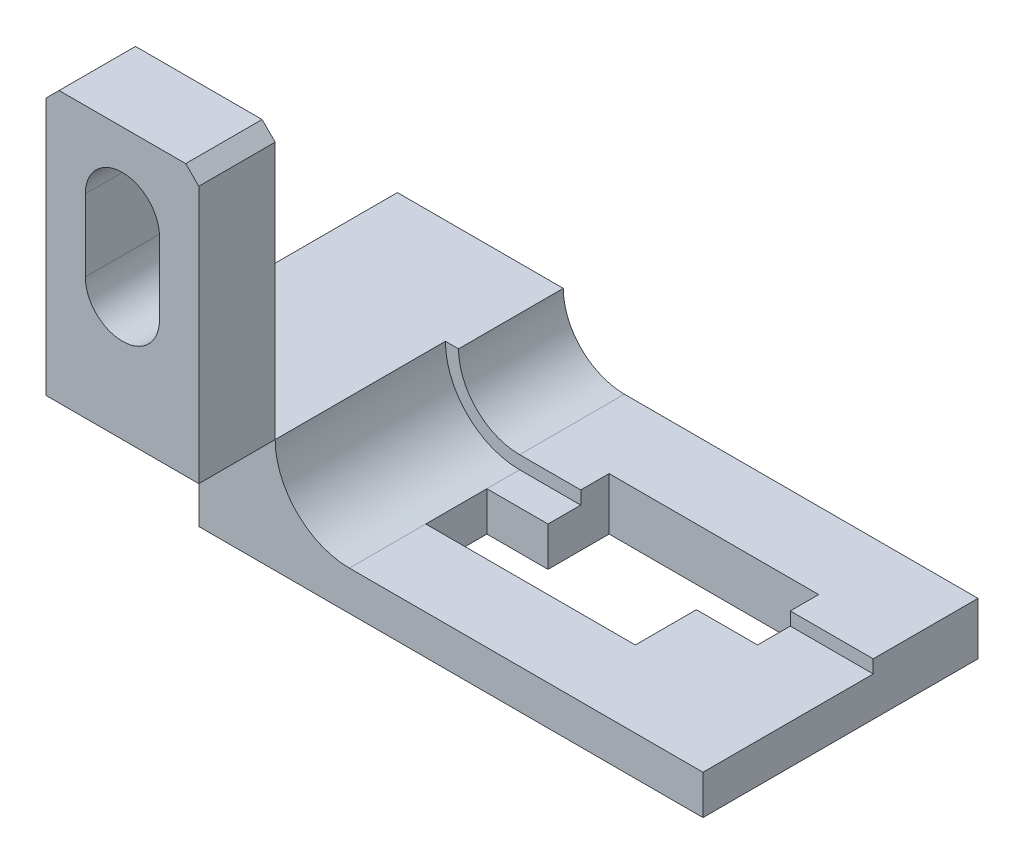
ISO-10303-21;
HEADER;
FILE_DESCRIPTION(('STEP AP214'),'2;1');
FILE_NAME('part.step','',(''),(''),'','','');
FILE_SCHEMA(('AUTOMOTIVE_DESIGN { 1 0 10303 214 1 1 1 1 }'));
ENDSEC;
DATA;
#1=APPLICATION_CONTEXT('core data for automotive mechanical design processes');
#2=APPLICATION_PROTOCOL_DEFINITION('international standard','automotive_design',2000,#1);
#3=PRODUCT_CONTEXT('',#1,'mechanical');
#4=PRODUCT('Part','Part','',(#3));
#5=PRODUCT_RELATED_PRODUCT_CATEGORY('part','',(#4));
#6=PRODUCT_DEFINITION_FORMATION('','',#4);
#7=PRODUCT_DEFINITION_CONTEXT('part definition',#1,'design');
#8=PRODUCT_DEFINITION('design','',#6,#7);
#9=PRODUCT_DEFINITION_SHAPE('','',#8);
#10=(LENGTH_UNIT() NAMED_UNIT(*) SI_UNIT(.MILLI.,.METRE.));
#11=(NAMED_UNIT(*) PLANE_ANGLE_UNIT() SI_UNIT($,.RADIAN.));
#12=(NAMED_UNIT(*) SI_UNIT($,.STERADIAN.) SOLID_ANGLE_UNIT());
#13=UNCERTAINTY_MEASURE_WITH_UNIT(LENGTH_MEASURE(1.E-05),#10,'distance_accuracy_value','');
#14=(GEOMETRIC_REPRESENTATION_CONTEXT(3) GLOBAL_UNCERTAINTY_ASSIGNED_CONTEXT((#13)) GLOBAL_UNIT_ASSIGNED_CONTEXT((#10,
#11,#12)) REPRESENTATION_CONTEXT('',''));
#15=CARTESIAN_POINT('',(0.,0.,0.));
#16=DIRECTION('',(0.,0.,1.));
#17=DIRECTION('',(1.,0.,0.));
#18=AXIS2_PLACEMENT_3D('',#15,#16,#17);
#19=CARTESIAN_POINT('',(0.,26.,80.5));
#20=DIRECTION('',(0.,1.,0.));
#21=DIRECTION('',(-1.,0.,0.));
#22=AXIS2_PLACEMENT_3D('',#19,#20,#21);
#23=PLANE('',#22);
#24=DIRECTION('',(1.,0.,0.));
#25=VECTOR('',#24,1.);
#26=CARTESIAN_POINT('',(0.,26.,63.));
#27=LINE('',#26,#25);
#28=CARTESIAN_POINT('',(-17.5,26.,63.));
#29=VERTEX_POINT('',#28);
#30=CARTESIAN_POINT('',(17.5,26.,63.));
#31=VERTEX_POINT('',#30);
#32=EDGE_CURVE('E165',#29,#31,#27,.T.);
#33=ORIENTED_EDGE('',*,*,#32,.T.);
#34=DIRECTION('',(0.,0.,-1.));
#35=VECTOR('',#34,1.);
#36=CARTESIAN_POINT('',(17.5,26.,80.5));
#37=LINE('',#36,#35);
#38=CARTESIAN_POINT('',(17.5,26.,80.5));
#39=VERTEX_POINT('',#38);
#40=EDGE_CURVE('E12',#39,#31,#37,.T.);
#41=ORIENTED_EDGE('',*,*,#40,.F.);
#42=DIRECTION('',(1.,0.,0.));
#43=VECTOR('',#42,1.);
#44=CARTESIAN_POINT('',(0.,26.,80.5));
#45=LINE('',#44,#43);
#46=CARTESIAN_POINT('',(-17.5,26.,80.5));
#47=VERTEX_POINT('',#46);
#48=EDGE_CURVE('E166',#47,#39,#45,.T.);
#49=ORIENTED_EDGE('',*,*,#48,.F.);
#50=DIRECTION('',(0.,0.,-1.));
#51=VECTOR('',#50,1.);
#52=CARTESIAN_POINT('',(-17.5,26.,80.5));
#53=LINE('',#52,#51);
#54=EDGE_CURVE('E181',#47,#29,#53,.T.);
#55=ORIENTED_EDGE('',*,*,#54,.T.);
#56=EDGE_LOOP('',(#33,#41,#49,#55));
#57=FACE_BOUND('',#56,.T.);
#58=ADVANCED_FACE('F54',(#57),#23,.F.);
#59=CARTESIAN_POINT('',(17.5,70.5,80.5));
#60=DIRECTION('',(-1.,0.,0.));
#61=DIRECTION('',(0.,0.,1.));
#62=AXIS2_PLACEMENT_3D('',#59,#60,#61);
#63=PLANE('',#62);
#64=DIRECTION('',(0.,1.,0.));
#65=VECTOR('',#64,1.);
#66=CARTESIAN_POINT('',(17.5,70.5,63.));
#67=LINE('',#66,#65);
#68=CARTESIAN_POINT('',(17.5,85.,63.));
#69=VERTEX_POINT('',#68);
#70=EDGE_CURVE('E183',#31,#69,#67,.T.);
#71=ORIENTED_EDGE('',*,*,#70,.T.);
#72=DIRECTION('',(0.,0.,-1.));
#73=VECTOR('',#72,1.);
#74=CARTESIAN_POINT('',(17.5,85.,80.5));
#75=LINE('',#74,#73);
#76=CARTESIAN_POINT('',(17.5,85.,80.5));
#77=VERTEX_POINT('',#76);
#78=EDGE_CURVE('E65',#77,#69,#75,.T.);
#79=ORIENTED_EDGE('',*,*,#78,.F.);
#80=DIRECTION('',(0.,1.,0.));
#81=VECTOR('',#80,1.);
#82=CARTESIAN_POINT('',(17.5,26.,80.5));
#83=LINE('',#82,#81);
#84=EDGE_CURVE('E167',#39,#77,#83,.T.);
#85=ORIENTED_EDGE('',*,*,#84,.F.);
#86=ORIENTED_EDGE('',*,*,#40,.T.);
#87=EDGE_LOOP('',(#71,#79,#85,#86));
#88=FACE_BOUND('',#87,.T.);
#89=ADVANCED_FACE('F229',(#88),#63,.F.);
#90=CARTESIAN_POINT('',(14.5,88.,80.5));
#91=DIRECTION('',(-0.707106781186548,-0.707106781186547,0.));
#92=DIRECTION('',(0.707106781186547,-0.707106781186548,0.));
#93=AXIS2_PLACEMENT_3D('',#90,#91,#92);
#94=PLANE('',#93);
#95=DIRECTION('',(-0.707106781186547,0.707106781186548,0.));
#96=VECTOR('',#95,1.);
#97=CARTESIAN_POINT('',(14.5,88.,63.));
#98=LINE('',#97,#96);
#99=CARTESIAN_POINT('',(14.5,88.,63.));
#100=VERTEX_POINT('',#99);
#101=EDGE_CURVE('E187',#69,#100,#98,.T.);
#102=ORIENTED_EDGE('',*,*,#101,.T.);
#103=DIRECTION('',(0.,0.,-1.));
#104=VECTOR('',#103,1.);
#105=CARTESIAN_POINT('',(14.5,88.,80.5));
#106=LINE('',#105,#104);
#107=CARTESIAN_POINT('',(14.5,88.,80.5));
#108=VERTEX_POINT('',#107);
#109=EDGE_CURVE('E204',#108,#100,#106,.T.);
#110=ORIENTED_EDGE('',*,*,#109,.F.);
#111=DIRECTION('',(-0.707106781186547,0.707106781186548,0.));
#112=VECTOR('',#111,1.);
#113=CARTESIAN_POINT('',(14.5,88.,80.5));
#114=LINE('',#113,#112);
#115=EDGE_CURVE('E173',#77,#108,#114,.T.);
#116=ORIENTED_EDGE('',*,*,#115,.F.);
#117=ORIENTED_EDGE('',*,*,#78,.T.);
#118=EDGE_LOOP('',(#102,#110,#116,#117));
#119=FACE_BOUND('',#118,.T.);
#120=ADVANCED_FACE('F208',(#119),#94,.F.);
#121=CARTESIAN_POINT('',(0.,88.,80.5));
#122=DIRECTION('',(0.,-1.,0.));
#123=DIRECTION('',(0.,0.,-1.));
#124=AXIS2_PLACEMENT_3D('',#121,#122,#123);
#125=PLANE('',#124);
#126=DIRECTION('',(-1.,0.,0.));
#127=VECTOR('',#126,1.);
#128=CARTESIAN_POINT('',(0.,88.,63.));
#129=LINE('',#128,#127);
#130=CARTESIAN_POINT('',(-14.5,88.,63.));
#131=VERTEX_POINT('',#130);
#132=EDGE_CURVE('E186',#100,#131,#129,.T.);
#133=ORIENTED_EDGE('',*,*,#132,.T.);
#134=DIRECTION('',(0.,0.,-1.));
#135=VECTOR('',#134,1.);
#136=CARTESIAN_POINT('',(-14.5,88.,80.5));
#137=LINE('',#136,#135);
#138=CARTESIAN_POINT('',(-14.5,88.,80.5));
#139=VERTEX_POINT('',#138);
#140=EDGE_CURVE('E198',#139,#131,#137,.T.);
#141=ORIENTED_EDGE('',*,*,#140,.F.);
#142=DIRECTION('',(-1.,0.,0.));
#143=VECTOR('',#142,1.);
#144=CARTESIAN_POINT('',(0.,88.,80.5));
#145=LINE('',#144,#143);
#146=EDGE_CURVE('E174',#108,#139,#145,.T.);
#147=ORIENTED_EDGE('',*,*,#146,.F.);
#148=ORIENTED_EDGE('',*,*,#109,.T.);
#149=EDGE_LOOP('',(#133,#141,#147,#148));
#150=FACE_BOUND('',#149,.T.);
#151=ADVANCED_FACE('F219',(#150),#125,.F.);
#152=CARTESIAN_POINT('',(-17.5,85.,80.5));
#153=DIRECTION('',(0.707106781186548,-0.707106781186547,0.));
#154=DIRECTION('',(0.707106781186547,0.707106781186548,0.));
#155=AXIS2_PLACEMENT_3D('',#152,#153,#154);
#156=PLANE('',#155);
#157=DIRECTION('',(-0.707106781186547,-0.707106781186548,0.));
#158=VECTOR('',#157,1.);
#159=CARTESIAN_POINT('',(-17.5,85.,63.));
#160=LINE('',#159,#158);
#161=CARTESIAN_POINT('',(-17.5,85.,63.));
#162=VERTEX_POINT('',#161);
#163=EDGE_CURVE('E192',#131,#162,#160,.T.);
#164=ORIENTED_EDGE('',*,*,#163,.T.);
#165=DIRECTION('',(0.,0.,-1.));
#166=VECTOR('',#165,1.);
#167=CARTESIAN_POINT('',(-17.5,85.,80.5));
#168=LINE('',#167,#166);
#169=CARTESIAN_POINT('',(-17.5,85.,80.5));
#170=VERTEX_POINT('',#169);
#171=EDGE_CURVE('E200',#170,#162,#168,.T.);
#172=ORIENTED_EDGE('',*,*,#171,.F.);
#173=DIRECTION('',(-0.707106781186547,-0.707106781186548,0.));
#174=VECTOR('',#173,1.);
#175=CARTESIAN_POINT('',(-17.5,85.,80.5));
#176=LINE('',#175,#174);
#177=EDGE_CURVE('E180',#139,#170,#176,.T.);
#178=ORIENTED_EDGE('',*,*,#177,.F.);
#179=ORIENTED_EDGE('',*,*,#140,.T.);
#180=EDGE_LOOP('',(#164,#172,#178,#179));
#181=FACE_BOUND('',#180,.T.);
#182=ADVANCED_FACE('F225',(#181),#156,.F.);
#183=CARTESIAN_POINT('',(-17.5,26.,80.5));
#184=DIRECTION('',(1.,0.,0.));
#185=DIRECTION('',(0.,0.,-1.));
#186=AXIS2_PLACEMENT_3D('',#183,#184,#185);
#187=PLANE('',#186);
#188=DIRECTION('',(0.,-1.,0.));
#189=VECTOR('',#188,1.);
#190=CARTESIAN_POINT('',(-17.5,26.,63.));
#191=LINE('',#190,#189);
#192=EDGE_CURVE('E171',#162,#29,#191,.T.);
#193=ORIENTED_EDGE('',*,*,#192,.T.);
#194=ORIENTED_EDGE('',*,*,#54,.F.);
#195=DIRECTION('',(0.,-1.,0.));
#196=VECTOR('',#195,1.);
#197=CARTESIAN_POINT('',(-17.5,26.,80.5));
#198=LINE('',#197,#196);
#199=EDGE_CURVE('E177',#170,#47,#198,.T.);
#200=ORIENTED_EDGE('',*,*,#199,.F.);
#201=ORIENTED_EDGE('',*,*,#171,.T.);
#202=EDGE_LOOP('',(#193,#194,#200,#201));
#203=FACE_BOUND('',#202,.T.);
#204=ADVANCED_FACE('F231',(#203),#187,.F.);
#205=CARTESIAN_POINT('',(0.,0.,80.5));
#206=DIRECTION('',(0.,0.,-1.));
#207=DIRECTION('',(-1.,0.,0.));
#208=AXIS2_PLACEMENT_3D('',#205,#206,#207);
#209=PLANE('',#208);
#210=DIRECTION('',(0.,-1.,0.));
#211=VECTOR('',#210,1.);
#212=CARTESIAN_POINT('',(-8.5,70.5,80.5));
#213=LINE('',#212,#211);
#214=CARTESIAN_POINT('',(-8.5,70.5,80.5));
#215=VERTEX_POINT('',#214);
#216=CARTESIAN_POINT('',(-8.5,54.,80.5));
#217=VERTEX_POINT('',#216);
#218=EDGE_CURVE('E159',#215,#217,#213,.T.);
#219=ORIENTED_EDGE('',*,*,#218,.F.);
#220=CARTESIAN_POINT('',(0.,70.5,80.5));
#221=DIRECTION('',(0.,0.,1.));
#222=DIRECTION('',(1.,0.,0.));
#223=AXIS2_PLACEMENT_3D('',#220,#221,#222);
#224=CIRCLE('',#223,8.5);
#225=CARTESIAN_POINT('',(8.5,70.5,80.5));
#226=VERTEX_POINT('',#225);
#227=EDGE_CURVE('E66',#226,#215,#224,.T.);
#228=ORIENTED_EDGE('',*,*,#227,.F.);
#229=DIRECTION('',(0.,1.,0.));
#230=VECTOR('',#229,1.);
#231=CARTESIAN_POINT('',(8.5,70.5,80.5));
#232=LINE('',#231,#230);
#233=CARTESIAN_POINT('',(8.5,54.,80.5));
#234=VERTEX_POINT('',#233);
#235=EDGE_CURVE('E146',#234,#226,#232,.T.);
#236=ORIENTED_EDGE('',*,*,#235,.F.);
#237=CARTESIAN_POINT('',(0.,54.,80.5));
#238=DIRECTION('',(0.,0.,1.));
#239=DIRECTION('',(1.,0.,0.));
#240=AXIS2_PLACEMENT_3D('',#237,#238,#239);
#241=CIRCLE('',#240,8.5);
#242=EDGE_CURVE('E155',#217,#234,#241,.T.);
#243=ORIENTED_EDGE('',*,*,#242,.F.);
#244=EDGE_LOOP('',(#219,#228,#236,#243));
#245=FACE_BOUND('',#244,.T.);
#246=ORIENTED_EDGE('',*,*,#48,.T.);
#247=ORIENTED_EDGE('',*,*,#84,.T.);
#248=ORIENTED_EDGE('',*,*,#115,.T.);
#249=ORIENTED_EDGE('',*,*,#146,.T.);
#250=ORIENTED_EDGE('',*,*,#177,.T.);
#251=ORIENTED_EDGE('',*,*,#199,.T.);
#252=EDGE_LOOP('',(#246,#247,#248,#249,#250,#251));
#253=FACE_BOUND('',#252,.T.);
#254=ADVANCED_FACE('F228',(#245,#253),#209,.F.);
#255=CARTESIAN_POINT('',(0.,0.,63.));
#256=DIRECTION('',(0.,0.,-1.));
#257=DIRECTION('',(-1.,0.,0.));
#258=AXIS2_PLACEMENT_3D('',#255,#256,#257);
#259=PLANE('',#258);
#260=CARTESIAN_POINT('',(0.,70.5,63.));
#261=DIRECTION('',(0.,0.,1.));
#262=DIRECTION('',(1.,0.,0.));
#263=AXIS2_PLACEMENT_3D('',#260,#261,#262);
#264=CIRCLE('',#263,8.5);
#265=CARTESIAN_POINT('',(8.5,70.5,63.));
#266=VERTEX_POINT('',#265);
#267=CARTESIAN_POINT('',(-8.5,70.5,63.));
#268=VERTEX_POINT('',#267);
#269=EDGE_CURVE('E134',#266,#268,#264,.T.);
#270=ORIENTED_EDGE('',*,*,#269,.T.);
#271=DIRECTION('',(0.,-1.,0.));
#272=VECTOR('',#271,1.);
#273=CARTESIAN_POINT('',(-8.5,70.5,63.));
#274=LINE('',#273,#272);
#275=CARTESIAN_POINT('',(-8.5,54.,63.));
#276=VERTEX_POINT('',#275);
#277=EDGE_CURVE('E145',#268,#276,#274,.T.);
#278=ORIENTED_EDGE('',*,*,#277,.T.);
#279=CARTESIAN_POINT('',(0.,54.,63.));
#280=DIRECTION('',(0.,0.,1.));
#281=DIRECTION('',(1.,0.,0.));
#282=AXIS2_PLACEMENT_3D('',#279,#280,#281);
#283=CIRCLE('',#282,8.5);
#284=CARTESIAN_POINT('',(8.5,54.,63.));
#285=VERTEX_POINT('',#284);
#286=EDGE_CURVE('E80',#276,#285,#283,.T.);
#287=ORIENTED_EDGE('',*,*,#286,.T.);
#288=DIRECTION('',(0.,1.,0.));
#289=VECTOR('',#288,1.);
#290=CARTESIAN_POINT('',(8.5,70.5,63.));
#291=LINE('',#290,#289);
#292=EDGE_CURVE('E136',#285,#266,#291,.T.);
#293=ORIENTED_EDGE('',*,*,#292,.T.);
#294=EDGE_LOOP('',(#270,#278,#287,#293));
#295=FACE_BOUND('',#294,.T.);
#296=ORIENTED_EDGE('',*,*,#32,.F.);
#297=ORIENTED_EDGE('',*,*,#192,.F.);
#298=ORIENTED_EDGE('',*,*,#163,.F.);
#299=ORIENTED_EDGE('',*,*,#132,.F.);
#300=ORIENTED_EDGE('',*,*,#101,.F.);
#301=ORIENTED_EDGE('',*,*,#70,.F.);
#302=EDGE_LOOP('',(#296,#297,#298,#299,#300,#301));
#303=FACE_BOUND('',#302,.T.);
#304=ADVANCED_FACE('F147',(#295,#303),#259,.T.);
#305=CARTESIAN_POINT('',(0.,70.5,63.));
#306=DIRECTION('',(0.,0.,1.));
#307=DIRECTION('',(1.,0.,0.));
#308=AXIS2_PLACEMENT_3D('',#305,#306,#307);
#309=CYLINDRICAL_SURFACE('',#308,8.5);
#310=ORIENTED_EDGE('',*,*,#227,.T.);
#311=DIRECTION('',(0.,0.,1.));
#312=VECTOR('',#311,1.);
#313=CARTESIAN_POINT('',(-8.5,70.5,63.));
#314=LINE('',#313,#312);
#315=EDGE_CURVE('E126',#268,#215,#314,.T.);
#316=ORIENTED_EDGE('',*,*,#315,.F.);
#317=ORIENTED_EDGE('',*,*,#269,.F.);
#318=DIRECTION('',(0.,0.,1.));
#319=VECTOR('',#318,1.);
#320=CARTESIAN_POINT('',(8.5,70.5,63.));
#321=LINE('',#320,#319);
#322=EDGE_CURVE('E162',#266,#226,#321,.T.);
#323=ORIENTED_EDGE('',*,*,#322,.T.);
#324=EDGE_LOOP('',(#310,#316,#317,#323));
#325=FACE_BOUND('',#324,.T.);
#326=ADVANCED_FACE('F132',(#325),#309,.F.);
#327=CARTESIAN_POINT('',(8.5,70.5,63.));
#328=DIRECTION('',(1.,0.,0.));
#329=DIRECTION('',(0.,1.,0.));
#330=AXIS2_PLACEMENT_3D('',#327,#328,#329);
#331=PLANE('',#330);
#332=ORIENTED_EDGE('',*,*,#235,.T.);
#333=ORIENTED_EDGE('',*,*,#322,.F.);
#334=ORIENTED_EDGE('',*,*,#292,.F.);
#335=DIRECTION('',(0.,0.,1.));
#336=VECTOR('',#335,1.);
#337=CARTESIAN_POINT('',(8.5,54.,63.));
#338=LINE('',#337,#336);
#339=EDGE_CURVE('E164',#285,#234,#338,.T.);
#340=ORIENTED_EDGE('',*,*,#339,.T.);
#341=EDGE_LOOP('',(#332,#333,#334,#340));
#342=FACE_BOUND('',#341,.T.);
#343=ADVANCED_FACE('F292',(#342),#331,.F.);
#344=CARTESIAN_POINT('',(0.,54.,63.));
#345=DIRECTION('',(0.,0.,1.));
#346=DIRECTION('',(1.,0.,0.));
#347=AXIS2_PLACEMENT_3D('',#344,#345,#346);
#348=CYLINDRICAL_SURFACE('',#347,8.5);
#349=ORIENTED_EDGE('',*,*,#242,.T.);
#350=ORIENTED_EDGE('',*,*,#339,.F.);
#351=ORIENTED_EDGE('',*,*,#286,.F.);
#352=DIRECTION('',(0.,0.,1.));
#353=VECTOR('',#352,1.);
#354=CARTESIAN_POINT('',(-8.5,54.,63.));
#355=LINE('',#354,#353);
#356=EDGE_CURVE('E139',#276,#217,#355,.T.);
#357=ORIENTED_EDGE('',*,*,#356,.T.);
#358=EDGE_LOOP('',(#349,#350,#351,#357));
#359=FACE_BOUND('',#358,.T.);
#360=ADVANCED_FACE('F303',(#359),#348,.F.);
#361=CARTESIAN_POINT('',(-8.5,70.5,63.));
#362=DIRECTION('',(-1.,0.,0.));
#363=DIRECTION('',(0.,-1.,0.));
#364=AXIS2_PLACEMENT_3D('',#361,#362,#363);
#365=PLANE('',#364);
#366=ORIENTED_EDGE('',*,*,#218,.T.);
#367=ORIENTED_EDGE('',*,*,#356,.F.);
#368=ORIENTED_EDGE('',*,*,#277,.F.);
#369=ORIENTED_EDGE('',*,*,#315,.T.);
#370=EDGE_LOOP('',(#366,#367,#368,#369));
#371=FACE_BOUND('',#370,.T.);
#372=ADVANCED_FACE('F141',(#371),#365,.F.);
#373=CLOSED_SHELL('',(#58,#89,#120,#151,#182,#204,#254,#304,#326,#343,#360,#372));
#374=MANIFOLD_SOLID_BREP('B2',#373);
#375=CARTESIAN_POINT('',(34.5,25.9999999999999,24.));
#376=DIRECTION('',(0.,0.,-1.));
#377=DIRECTION('',(-1.,0.,0.));
#378=AXIS2_PLACEMENT_3D('',#375,#376,#377);
#379=PLANE('',#378);
#380=DIRECTION('',(-1.,0.,0.));
#381=VECTOR('',#380,1.);
#382=CARTESIAN_POINT('',(115.5,8.99999999999991,24.));
#383=LINE('',#382,#381);
#384=CARTESIAN_POINT('',(48.5,8.9999999999999,24.));
#385=VERTEX_POINT('',#384);
#386=CARTESIAN_POINT('',(34.4999999999998,8.9999999999999,24.));
#387=VERTEX_POINT('',#386);
#388=EDGE_CURVE('E556',#385,#387,#383,.T.);
#389=ORIENTED_EDGE('',*,*,#388,.F.);
#390=DIRECTION('',(0.,-1.,0.));
#391=VECTOR('',#390,1.);
#392=CARTESIAN_POINT('',(48.5,11.9999999999999,24.));
#393=LINE('',#392,#391);
#394=CARTESIAN_POINT('',(48.5,11.9999999999999,24.));
#395=VERTEX_POINT('',#394);
#396=EDGE_CURVE('E538',#395,#385,#393,.T.);
#397=ORIENTED_EDGE('',*,*,#396,.F.);
#398=DIRECTION('',(1.,0.,0.));
#399=VECTOR('',#398,1.);
#400=CARTESIAN_POINT('',(34.5,11.9999999999999,24.));
#401=LINE('',#400,#399);
#402=CARTESIAN_POINT('',(34.5,11.9999999999999,24.));
#403=VERTEX_POINT('',#402);
#404=EDGE_CURVE('E533',#403,#395,#401,.T.);
#405=ORIENTED_EDGE('',*,*,#404,.F.);
#406=CARTESIAN_POINT('',(34.5,25.9999999999999,24.));
#407=DIRECTION('',(0.,0.,1.));
#408=DIRECTION('',(-1.,0.,0.));
#409=AXIS2_PLACEMENT_3D('',#406,#407,#408);
#410=CIRCLE('',#409,14.);
#411=CARTESIAN_POINT('',(20.5,25.9999999999999,24.));
#412=VERTEX_POINT('',#411);
#413=EDGE_CURVE('E553',#412,#403,#410,.T.);
#414=ORIENTED_EDGE('',*,*,#413,.F.);
#415=DIRECTION('',(1.,0.,0.));
#416=VECTOR('',#415,1.);
#417=CARTESIAN_POINT('',(17.5,26.,24.));
#418=LINE('',#417,#416);
#419=CARTESIAN_POINT('',(17.5,26.,24.));
#420=VERTEX_POINT('',#419);
#421=EDGE_CURVE('E550',#420,#412,#418,.T.);
#422=ORIENTED_EDGE('',*,*,#421,.F.);
#423=CARTESIAN_POINT('',(34.5,25.9999999999999,24.));
#424=DIRECTION('',(0.,0.,-1.));
#425=DIRECTION('',(-1.,0.,0.));
#426=AXIS2_PLACEMENT_3D('',#423,#424,#425);
#427=CIRCLE('',#426,17.);
#428=EDGE_CURVE('E541',#387,#420,#427,.T.);
#429=ORIENTED_EDGE('',*,*,#428,.F.);
#430=EDGE_LOOP('',(#389,#397,#405,#414,#422,#429));
#431=FACE_BOUND('',#430,.T.);
#432=ADVANCED_FACE('F362',(#431),#379,.F.);
#433=CARTESIAN_POINT('',(115.5,8.99999999999991,63.));
#434=DIRECTION('',(0.,-1.,0.));
#435=DIRECTION('',(1.,0.,0.));
#436=AXIS2_PLACEMENT_3D('',#433,#434,#435);
#437=PLANE('',#436);
#438=ORIENTED_EDGE('',*,*,#388,.T.);
#439=DIRECTION('',(0.,0.,-1.));
#440=VECTOR('',#439,1.);
#441=CARTESIAN_POINT('',(34.5,8.9999999999999,63.));
#442=LINE('',#441,#440);
#443=CARTESIAN_POINT('',(34.5,8.9999999999999,31.5));
#444=VERTEX_POINT('',#443);
#445=EDGE_CURVE('E671',#444,#387,#442,.T.);
#446=ORIENTED_EDGE('',*,*,#445,.F.);
#447=DIRECTION('',(-1.,0.,0.));
#448=VECTOR('',#447,1.);
#449=CARTESIAN_POINT('',(48.5,8.9999999999999,31.5));
#450=LINE('',#449,#448);
#451=CARTESIAN_POINT('',(48.5,8.9999999999999,31.5));
#452=VERTEX_POINT('',#451);
#453=EDGE_CURVE('E389',#452,#444,#450,.T.);
#454=ORIENTED_EDGE('',*,*,#453,.F.);
#455=DIRECTION('',(0.,0.,1.));
#456=VECTOR('',#455,1.);
#457=CARTESIAN_POINT('',(48.5,8.9999999999999,17.5));
#458=LINE('',#457,#456);
#459=EDGE_CURVE('E599',#385,#452,#458,.T.);
#460=ORIENTED_EDGE('',*,*,#459,.F.);
#461=EDGE_LOOP('',(#438,#446,#454,#460));
#462=FACE_BOUND('',#461,.T.);
#463=ADVANCED_FACE('F745',(#462),#437,.F.);
#464=CARTESIAN_POINT('',(115.5,8.99999999999991,24.));
#465=VERTEX_POINT('',#464);
#466=CARTESIAN_POINT('',(96.5,8.99999999999991,24.));
#467=VERTEX_POINT('',#466);
#468=EDGE_CURVE('E559',#465,#467,#383,.T.);
#469=ORIENTED_EDGE('',*,*,#468,.T.);
#470=DIRECTION('',(0.,0.,-1.));
#471=VECTOR('',#470,1.);
#472=CARTESIAN_POINT('',(96.5,8.99999999999991,17.5));
#473=LINE('',#472,#471);
#474=CARTESIAN_POINT('',(96.5,8.99999999999991,31.5));
#475=VERTEX_POINT('',#474);
#476=EDGE_CURVE('E569',#475,#467,#473,.T.);
#477=ORIENTED_EDGE('',*,*,#476,.F.);
#478=DIRECTION('',(1.,0.,0.));
#479=VECTOR('',#478,1.);
#480=CARTESIAN_POINT('',(96.5,8.99999999999991,31.5));
#481=LINE('',#480,#479);
#482=CARTESIAN_POINT('',(82.5,8.9999999999999,31.5));
#483=VERTEX_POINT('',#482);
#484=EDGE_CURVE('E576',#483,#475,#481,.T.);
#485=ORIENTED_EDGE('',*,*,#484,.F.);
#486=DIRECTION('',(0.,0.,-1.));
#487=VECTOR('',#486,1.);
#488=CARTESIAN_POINT('',(82.5,8.9999999999999,31.5));
#489=LINE('',#488,#487);
#490=CARTESIAN_POINT('',(82.5,8.9999999999999,45.5));
#491=VERTEX_POINT('',#490);
#492=EDGE_CURVE('E609',#491,#483,#489,.T.);
#493=ORIENTED_EDGE('',*,*,#492,.F.);
#494=DIRECTION('',(1.,0.,0.));
#495=VECTOR('',#494,1.);
#496=CARTESIAN_POINT('',(82.5,8.9999999999999,45.5));
#497=LINE('',#496,#495);
#498=CARTESIAN_POINT('',(34.5,8.9999999999999,45.5));
#499=VERTEX_POINT('',#498);
#500=EDGE_CURVE('E603',#499,#491,#497,.T.);
#501=ORIENTED_EDGE('',*,*,#500,.F.);
#502=CARTESIAN_POINT('',(34.5,8.9999999999999,63.));
#503=VERTEX_POINT('',#502);
#504=EDGE_CURVE('E673',#503,#499,#442,.T.);
#505=ORIENTED_EDGE('',*,*,#504,.F.);
#506=DIRECTION('',(-1.,0.,0.));
#507=VECTOR('',#506,1.);
#508=CARTESIAN_POINT('',(115.5,8.99999999999991,63.));
#509=LINE('',#508,#507);
#510=CARTESIAN_POINT('',(115.5,8.99999999999991,63.));
#511=VERTEX_POINT('',#510);
#512=EDGE_CURVE('E632',#511,#503,#509,.T.);
#513=ORIENTED_EDGE('',*,*,#512,.F.);
#514=DIRECTION('',(0.,0.,-1.));
#515=VECTOR('',#514,1.);
#516=CARTESIAN_POINT('',(115.5,8.99999999999991,63.));
#517=LINE('',#516,#515);
#518=EDGE_CURVE('E679',#511,#465,#517,.T.);
#519=ORIENTED_EDGE('',*,*,#518,.T.);
#520=EDGE_LOOP('',(#469,#477,#485,#493,#501,#505,#513,#519));
#521=FACE_BOUND('',#520,.T.);
#522=ADVANCED_FACE('F705',(#521),#437,.F.);
#523=CARTESIAN_POINT('',(34.5,25.9999999999999,63.));
#524=DIRECTION('',(0.,0.,-1.));
#525=DIRECTION('',(-1.,0.,0.));
#526=AXIS2_PLACEMENT_3D('',#523,#524,#525);
#527=CYLINDRICAL_SURFACE('',#526,17.);
#528=ORIENTED_EDGE('',*,*,#428,.T.);
#529=DIRECTION('',(0.,0.,-1.));
#530=VECTOR('',#529,1.);
#531=CARTESIAN_POINT('',(17.5,26.,63.));
#532=LINE('',#531,#530);
#533=CARTESIAN_POINT('',(17.5,26.,63.));
#534=VERTEX_POINT('',#533);
#535=EDGE_CURVE('E672',#534,#420,#532,.T.);
#536=ORIENTED_EDGE('',*,*,#535,.F.);
#537=CARTESIAN_POINT('',(34.5,25.9999999999999,63.));
#538=DIRECTION('',(0.,0.,-1.));
#539=DIRECTION('',(1.,0.,0.));
#540=AXIS2_PLACEMENT_3D('',#537,#538,#539);
#541=CIRCLE('',#540,17.);
#542=EDGE_CURVE('E636',#503,#534,#541,.T.);
#543=ORIENTED_EDGE('',*,*,#542,.F.);
#544=ORIENTED_EDGE('',*,*,#504,.T.);
#545=DIRECTION('',(0.,0.,1.));
#546=VECTOR('',#545,1.);
#547=CARTESIAN_POINT('',(34.5,8.9999999999999,45.5));
#548=LINE('',#547,#546);
#549=EDGE_CURVE('E605',#444,#499,#548,.T.);
#550=ORIENTED_EDGE('',*,*,#549,.F.);
#551=ORIENTED_EDGE('',*,*,#445,.T.);
#552=EDGE_LOOP('',(#528,#536,#543,#544,#550,#551));
#553=FACE_BOUND('',#552,.T.);
#554=ADVANCED_FACE('F748',(#553),#527,.F.);
#555=CARTESIAN_POINT('',(0.,0.,63.));
#556=DIRECTION('',(1.,0.,0.));
#557=DIRECTION('',(0.,0.,-1.));
#558=AXIS2_PLACEMENT_3D('',#555,#556,#557);
#559=PLANE('',#558);
#560=DIRECTION('',(0.,-1.,0.));
#561=VECTOR('',#560,1.);
#562=CARTESIAN_POINT('',(0.,0.,0.));
#563=LINE('',#562,#561);
#564=CARTESIAN_POINT('',(0.,16.5,0.));
#565=VERTEX_POINT('',#564);
#566=CARTESIAN_POINT('',(0.,0.,0.));
#567=VERTEX_POINT('',#566);
#568=EDGE_CURVE('E613',#565,#567,#563,.T.);
#569=ORIENTED_EDGE('',*,*,#568,.T.);
#570=DIRECTION('',(0.,0.,-1.));
#571=VECTOR('',#570,1.);
#572=CARTESIAN_POINT('',(0.,0.,63.));
#573=LINE('',#572,#571);
#574=CARTESIAN_POINT('',(0.,0.,63.));
#575=VERTEX_POINT('',#574);
#576=EDGE_CURVE('E52',#575,#567,#573,.T.);
#577=ORIENTED_EDGE('',*,*,#576,.F.);
#578=DIRECTION('',(0.,-1.,0.));
#579=VECTOR('',#578,1.);
#580=CARTESIAN_POINT('',(0.,0.,63.));
#581=LINE('',#580,#579);
#582=CARTESIAN_POINT('',(0.,16.5,63.));
#583=VERTEX_POINT('',#582);
#584=EDGE_CURVE('E626',#583,#575,#581,.T.);
#585=ORIENTED_EDGE('',*,*,#584,.F.);
#586=DIRECTION('',(0.,0.,-1.));
#587=VECTOR('',#586,1.);
#588=CARTESIAN_POINT('',(0.,16.5,63.));
#589=LINE('',#588,#587);
#590=EDGE_CURVE('E647',#583,#565,#589,.T.);
#591=ORIENTED_EDGE('',*,*,#590,.T.);
#592=EDGE_LOOP('',(#569,#577,#585,#591));
#593=FACE_BOUND('',#592,.T.);
#594=ADVANCED_FACE('F370',(#593),#559,.F.);
#595=CARTESIAN_POINT('',(0.,0.,63.));
#596=DIRECTION('',(0.,1.,0.));
#597=DIRECTION('',(0.,0.,1.));
#598=AXIS2_PLACEMENT_3D('',#595,#596,#597);
#599=PLANE('',#598);
#600=DIRECTION('',(1.,0.,0.));
#601=VECTOR('',#600,1.);
#602=CARTESIAN_POINT('',(96.5,0.,31.5));
#603=LINE('',#602,#601);
#604=CARTESIAN_POINT('',(82.5,0.,31.5));
#605=VERTEX_POINT('',#604);
#606=CARTESIAN_POINT('',(96.5,0.,31.5));
#607=VERTEX_POINT('',#606);
#608=EDGE_CURVE('E591',#605,#607,#603,.T.);
#609=ORIENTED_EDGE('',*,*,#608,.T.);
#610=DIRECTION('',(0.,0.,-1.));
#611=VECTOR('',#610,1.);
#612=CARTESIAN_POINT('',(96.5,0.,17.5));
#613=LINE('',#612,#611);
#614=CARTESIAN_POINT('',(96.5,0.,17.5));
#615=VERTEX_POINT('',#614);
#616=EDGE_CURVE('E574',#607,#615,#613,.T.);
#617=ORIENTED_EDGE('',*,*,#616,.T.);
#618=DIRECTION('',(-1.,0.,0.));
#619=VECTOR('',#618,1.);
#620=CARTESIAN_POINT('',(96.5,0.,17.5));
#621=LINE('',#620,#619);
#622=CARTESIAN_POINT('',(48.5,0.,17.5));
#623=VERTEX_POINT('',#622);
#624=EDGE_CURVE('E579',#615,#623,#621,.T.);
#625=ORIENTED_EDGE('',*,*,#624,.T.);
#626=DIRECTION('',(0.,0.,1.));
#627=VECTOR('',#626,1.);
#628=CARTESIAN_POINT('',(48.5,0.,17.5));
#629=LINE('',#628,#627);
#630=CARTESIAN_POINT('',(48.5,0.,31.5));
#631=VERTEX_POINT('',#630);
#632=EDGE_CURVE('E379',#623,#631,#629,.T.);
#633=ORIENTED_EDGE('',*,*,#632,.T.);
#634=DIRECTION('',(-1.,0.,0.));
#635=VECTOR('',#634,1.);
#636=CARTESIAN_POINT('',(48.5,0.,31.5));
#637=LINE('',#636,#635);
#638=CARTESIAN_POINT('',(34.5,0.,31.5));
#639=VERTEX_POINT('',#638);
#640=EDGE_CURVE('E585',#631,#639,#637,.T.);
#641=ORIENTED_EDGE('',*,*,#640,.T.);
#642=DIRECTION('',(0.,0.,1.));
#643=VECTOR('',#642,1.);
#644=CARTESIAN_POINT('',(34.5,0.,45.5));
#645=LINE('',#644,#643);
#646=CARTESIAN_POINT('',(34.5,0.,45.5));
#647=VERTEX_POINT('',#646);
#648=EDGE_CURVE('E583',#639,#647,#645,.T.);
#649=ORIENTED_EDGE('',*,*,#648,.T.);
#650=DIRECTION('',(1.,0.,0.));
#651=VECTOR('',#650,1.);
#652=CARTESIAN_POINT('',(82.5,0.,45.5));
#653=LINE('',#652,#651);
#654=CARTESIAN_POINT('',(82.5,0.,45.5));
#655=VERTEX_POINT('',#654);
#656=EDGE_CURVE('E589',#647,#655,#653,.T.);
#657=ORIENTED_EDGE('',*,*,#656,.T.);
#658=DIRECTION('',(0.,0.,-1.));
#659=VECTOR('',#658,1.);
#660=CARTESIAN_POINT('',(82.5,0.,31.5));
#661=LINE('',#660,#659);
#662=EDGE_CURVE('E592',#655,#605,#661,.T.);
#663=ORIENTED_EDGE('',*,*,#662,.T.);
#664=EDGE_LOOP('',(#609,#617,#625,#633,#641,#649,#657,#663));
#665=FACE_BOUND('',#664,.T.);
#666=DIRECTION('',(1.,0.,0.));
#667=VECTOR('',#666,1.);
#668=CARTESIAN_POINT('',(0.,0.,0.));
#669=LINE('',#668,#667);
#670=CARTESIAN_POINT('',(115.5,0.,0.));
#671=VERTEX_POINT('',#670);
#672=EDGE_CURVE('E646',#567,#671,#669,.T.);
#673=ORIENTED_EDGE('',*,*,#672,.T.);
#674=DIRECTION('',(0.,0.,-1.));
#675=VECTOR('',#674,1.);
#676=CARTESIAN_POINT('',(115.5,0.,63.));
#677=LINE('',#676,#675);
#678=CARTESIAN_POINT('',(115.5,0.,63.));
#679=VERTEX_POINT('',#678);
#680=EDGE_CURVE('E373',#679,#671,#677,.T.);
#681=ORIENTED_EDGE('',*,*,#680,.F.);
#682=DIRECTION('',(1.,0.,0.));
#683=VECTOR('',#682,1.);
#684=CARTESIAN_POINT('',(0.,0.,63.));
#685=LINE('',#684,#683);
#686=EDGE_CURVE('E627',#575,#679,#685,.T.);
#687=ORIENTED_EDGE('',*,*,#686,.F.);
#688=ORIENTED_EDGE('',*,*,#576,.T.);
#689=EDGE_LOOP('',(#673,#681,#687,#688));
#690=FACE_BOUND('',#689,.T.);
#691=ADVANCED_FACE('F712',(#665,#690),#599,.F.);
#692=CARTESIAN_POINT('',(115.5,8.99999999999991,63.));
#693=DIRECTION('',(-1.,0.,0.));
#694=DIRECTION('',(0.,-1.,0.));
#695=AXIS2_PLACEMENT_3D('',#692,#693,#694);
#696=PLANE('',#695);
#697=DIRECTION('',(0.,1.,0.));
#698=VECTOR('',#697,1.);
#699=CARTESIAN_POINT('',(115.5,8.99999999999991,0.));
#700=LINE('',#699,#698);
#701=CARTESIAN_POINT('',(115.5,11.9999999999999,0.));
#702=VERTEX_POINT('',#701);
#703=EDGE_CURVE('E652',#671,#702,#700,.T.);
#704=ORIENTED_EDGE('',*,*,#703,.T.);
#705=DIRECTION('',(0.,0.,-1.));
#706=VECTOR('',#705,1.);
#707=CARTESIAN_POINT('',(115.5,11.9999999999999,24.));
#708=LINE('',#707,#706);
#709=CARTESIAN_POINT('',(115.5,11.9999999999999,24.));
#710=VERTEX_POINT('',#709);
#711=EDGE_CURVE('E570',#710,#702,#708,.T.);
#712=ORIENTED_EDGE('',*,*,#711,.F.);
#713=DIRECTION('',(0.,-1.,0.));
#714=VECTOR('',#713,1.);
#715=CARTESIAN_POINT('',(115.5,11.9999999999999,24.));
#716=LINE('',#715,#714);
#717=EDGE_CURVE('E558',#710,#465,#716,.T.);
#718=ORIENTED_EDGE('',*,*,#717,.T.);
#719=ORIENTED_EDGE('',*,*,#518,.F.);
#720=DIRECTION('',(0.,1.,0.));
#721=VECTOR('',#720,1.);
#722=CARTESIAN_POINT('',(115.5,8.99999999999991,63.));
#723=LINE('',#722,#721);
#724=EDGE_CURVE('E635',#679,#511,#723,.T.);
#725=ORIENTED_EDGE('',*,*,#724,.F.);
#726=ORIENTED_EDGE('',*,*,#680,.T.);
#727=EDGE_LOOP('',(#704,#712,#718,#719,#725,#726));
#728=FACE_BOUND('',#727,.T.);
#729=ADVANCED_FACE('F684',(#728),#696,.F.);
#730=CARTESIAN_POINT('',(17.5,26.,63.));
#731=DIRECTION('',(0.,-1.,0.));
#732=DIRECTION('',(1.,0.,0.));
#733=AXIS2_PLACEMENT_3D('',#730,#731,#732);
#734=PLANE('',#733);
#735=DIRECTION('',(-1.,0.,0.));
#736=VECTOR('',#735,1.);
#737=CARTESIAN_POINT('',(17.5,26.,0.));
#738=LINE('',#737,#736);
#739=CARTESIAN_POINT('',(20.5,25.9999999999999,0.));
#740=VERTEX_POINT('',#739);
#741=CARTESIAN_POINT('',(-17.5,26.,0.));
#742=VERTEX_POINT('',#741);
#743=EDGE_CURVE('E654',#740,#742,#738,.T.);
#744=ORIENTED_EDGE('',*,*,#743,.T.);
#745=DIRECTION('',(0.,0.,-1.));
#746=VECTOR('',#745,1.);
#747=CARTESIAN_POINT('',(-17.5,26.,63.));
#748=LINE('',#747,#746);
#749=CARTESIAN_POINT('',(-17.5,26.,63.));
#750=VERTEX_POINT('',#749);
#751=EDGE_CURVE('E669',#750,#742,#748,.T.);
#752=ORIENTED_EDGE('',*,*,#751,.F.);
#753=DIRECTION('',(-1.,0.,0.));
#754=VECTOR('',#753,1.);
#755=CARTESIAN_POINT('',(17.5,26.,63.));
#756=LINE('',#755,#754);
#757=EDGE_CURVE('E637',#534,#750,#756,.T.);
#758=ORIENTED_EDGE('',*,*,#757,.F.);
#759=ORIENTED_EDGE('',*,*,#535,.T.);
#760=ORIENTED_EDGE('',*,*,#421,.T.);
#761=DIRECTION('',(0.,0.,-1.));
#762=VECTOR('',#761,1.);
#763=CARTESIAN_POINT('',(20.5,25.9999999999999,24.));
#764=LINE('',#763,#762);
#765=EDGE_CURVE('E565',#412,#740,#764,.T.);
#766=ORIENTED_EDGE('',*,*,#765,.T.);
#767=EDGE_LOOP('',(#744,#752,#758,#759,#760,#766));
#768=FACE_BOUND('',#767,.T.);
#769=ADVANCED_FACE('F728',(#768),#734,.F.);
#770=CARTESIAN_POINT('',(-17.5,26.,63.));
#771=DIRECTION('',(1.,0.,0.));
#772=DIRECTION('',(0.,0.,-1.));
#773=AXIS2_PLACEMENT_3D('',#770,#771,#772);
#774=PLANE('',#773);
#775=DIRECTION('',(0.,-1.,0.));
#776=VECTOR('',#775,1.);
#777=CARTESIAN_POINT('',(-17.5,26.,0.));
#778=LINE('',#777,#776);
#779=CARTESIAN_POINT('',(-17.5,20.,0.));
#780=VERTEX_POINT('',#779);
#781=EDGE_CURVE('E653',#742,#780,#778,.T.);
#782=ORIENTED_EDGE('',*,*,#781,.T.);
#783=DIRECTION('',(0.,0.,-1.));
#784=VECTOR('',#783,1.);
#785=CARTESIAN_POINT('',(-17.5,20.,63.));
#786=LINE('',#785,#784);
#787=CARTESIAN_POINT('',(-17.5,20.,63.));
#788=VERTEX_POINT('',#787);
#789=EDGE_CURVE('E663',#788,#780,#786,.T.);
#790=ORIENTED_EDGE('',*,*,#789,.F.);
#791=DIRECTION('',(0.,-1.,0.));
#792=VECTOR('',#791,1.);
#793=CARTESIAN_POINT('',(-17.5,26.,63.));
#794=LINE('',#793,#792);
#795=EDGE_CURVE('E639',#750,#788,#794,.T.);
#796=ORIENTED_EDGE('',*,*,#795,.F.);
#797=ORIENTED_EDGE('',*,*,#751,.T.);
#798=EDGE_LOOP('',(#782,#790,#796,#797));
#799=FACE_BOUND('',#798,.T.);
#800=ADVANCED_FACE('F730',(#799),#774,.F.);
#801=CARTESIAN_POINT('',(-3.50000000000002,20.,63.));
#802=DIRECTION('',(0.,1.,0.));
#803=DIRECTION('',(0.,0.,1.));
#804=AXIS2_PLACEMENT_3D('',#801,#802,#803);
#805=PLANE('',#804);
#806=DIRECTION('',(1.,0.,0.));
#807=VECTOR('',#806,1.);
#808=CARTESIAN_POINT('',(-3.50000000000002,20.,0.));
#809=LINE('',#808,#807);
#810=CARTESIAN_POINT('',(-3.50000000000002,20.,0.));
#811=VERTEX_POINT('',#810);
#812=EDGE_CURVE('E660',#780,#811,#809,.T.);
#813=ORIENTED_EDGE('',*,*,#812,.T.);
#814=DIRECTION('',(0.,0.,-1.));
#815=VECTOR('',#814,1.);
#816=CARTESIAN_POINT('',(-3.50000000000002,20.,63.));
#817=LINE('',#816,#815);
#818=CARTESIAN_POINT('',(-3.50000000000002,20.,63.));
#819=VERTEX_POINT('',#818);
#820=EDGE_CURVE('E665',#819,#811,#817,.T.);
#821=ORIENTED_EDGE('',*,*,#820,.F.);
#822=DIRECTION('',(1.,0.,0.));
#823=VECTOR('',#822,1.);
#824=CARTESIAN_POINT('',(-3.50000000000002,20.,63.));
#825=LINE('',#824,#823);
#826=EDGE_CURVE('E645',#788,#819,#825,.T.);
#827=ORIENTED_EDGE('',*,*,#826,.F.);
#828=ORIENTED_EDGE('',*,*,#789,.T.);
#829=EDGE_LOOP('',(#813,#821,#827,#828));
#830=FACE_BOUND('',#829,.T.);
#831=ADVANCED_FACE('F724',(#830),#805,.F.);
#832=CARTESIAN_POINT('',(-3.5,16.5,63.));
#833=DIRECTION('',(0.,0.,-1.));
#834=DIRECTION('',(-1.,0.,0.));
#835=AXIS2_PLACEMENT_3D('',#832,#833,#834);
#836=CYLINDRICAL_SURFACE('',#835,3.5);
#837=CARTESIAN_POINT('',(-3.5,16.5,0.));
#838=DIRECTION('',(0.,0.,-1.));
#839=DIRECTION('',(-1.,0.,0.));
#840=AXIS2_PLACEMENT_3D('',#837,#838,#839);
#841=CIRCLE('',#840,3.5);
#842=EDGE_CURVE('E629',#811,#565,#841,.T.);
#843=ORIENTED_EDGE('',*,*,#842,.T.);
#844=ORIENTED_EDGE('',*,*,#590,.F.);
#845=CARTESIAN_POINT('',(-3.5,16.5,63.));
#846=DIRECTION('',(0.,0.,-1.));
#847=DIRECTION('',(-1.,0.,0.));
#848=AXIS2_PLACEMENT_3D('',#845,#846,#847);
#849=CIRCLE('',#848,3.5);
#850=EDGE_CURVE('E641',#819,#583,#849,.T.);
#851=ORIENTED_EDGE('',*,*,#850,.F.);
#852=ORIENTED_EDGE('',*,*,#820,.T.);
#853=EDGE_LOOP('',(#843,#844,#851,#852));
#854=FACE_BOUND('',#853,.T.);
#855=ADVANCED_FACE('F719',(#854),#836,.F.);
#856=CARTESIAN_POINT('',(-3.5,16.5,63.));
#857=DIRECTION('',(0.,0.,-1.));
#858=DIRECTION('',(-1.,0.,0.));
#859=AXIS2_PLACEMENT_3D('',#856,#857,#858);
#860=PLANE('',#859);
#861=ORIENTED_EDGE('',*,*,#584,.T.);
#862=ORIENTED_EDGE('',*,*,#686,.T.);
#863=ORIENTED_EDGE('',*,*,#724,.T.);
#864=ORIENTED_EDGE('',*,*,#512,.T.);
#865=ORIENTED_EDGE('',*,*,#542,.T.);
#866=ORIENTED_EDGE('',*,*,#757,.T.);
#867=ORIENTED_EDGE('',*,*,#795,.T.);
#868=ORIENTED_EDGE('',*,*,#826,.T.);
#869=ORIENTED_EDGE('',*,*,#850,.T.);
#870=EDGE_LOOP('',(#861,#862,#863,#864,#865,#866,#867,#868,#869));
#871=FACE_BOUND('',#870,.T.);
#872=ADVANCED_FACE('F710',(#871),#860,.F.);
#873=CARTESIAN_POINT('',(-3.5,16.5,0.));
#874=DIRECTION('',(0.,0.,-1.));
#875=DIRECTION('',(-1.,0.,0.));
#876=AXIS2_PLACEMENT_3D('',#873,#874,#875);
#877=PLANE('',#876);
#878=ORIENTED_EDGE('',*,*,#743,.F.);
#879=CARTESIAN_POINT('',(34.5,25.9999999999999,0.));
#880=DIRECTION('',(0.,0.,1.));
#881=DIRECTION('',(-1.,0.,0.));
#882=AXIS2_PLACEMENT_3D('',#879,#880,#881);
#883=CIRCLE('',#882,14.);
#884=CARTESIAN_POINT('',(34.5,11.9999999999999,0.));
#885=VERTEX_POINT('',#884);
#886=EDGE_CURVE('E545',#740,#885,#883,.T.);
#887=ORIENTED_EDGE('',*,*,#886,.T.);
#888=DIRECTION('',(1.,0.,0.));
#889=VECTOR('',#888,1.);
#890=CARTESIAN_POINT('',(34.5,11.9999999999999,0.));
#891=LINE('',#890,#889);
#892=EDGE_CURVE('E549',#885,#702,#891,.T.);
#893=ORIENTED_EDGE('',*,*,#892,.T.);
#894=ORIENTED_EDGE('',*,*,#703,.F.);
#895=ORIENTED_EDGE('',*,*,#672,.F.);
#896=ORIENTED_EDGE('',*,*,#568,.F.);
#897=ORIENTED_EDGE('',*,*,#842,.F.);
#898=ORIENTED_EDGE('',*,*,#812,.F.);
#899=ORIENTED_EDGE('',*,*,#781,.F.);
#900=EDGE_LOOP('',(#878,#887,#893,#894,#895,#896,#897,#898,#899));
#901=FACE_BOUND('',#900,.T.);
#902=ADVANCED_FACE('F687',(#901),#877,.T.);
#903=CARTESIAN_POINT('',(96.5,0.,17.5));
#904=DIRECTION('',(1.,0.,0.));
#905=DIRECTION('',(0.,1.,0.));
#906=AXIS2_PLACEMENT_3D('',#903,#904,#905);
#907=PLANE('',#906);
#908=ORIENTED_EDGE('',*,*,#476,.T.);
#909=DIRECTION('',(0.,-1.,0.));
#910=VECTOR('',#909,1.);
#911=CARTESIAN_POINT('',(96.5,11.9999999999999,24.));
#912=LINE('',#911,#910);
#913=CARTESIAN_POINT('',(96.5,11.9999999999999,24.));
#914=VERTEX_POINT('',#913);
#915=EDGE_CURVE('E536',#914,#467,#912,.T.);
#916=ORIENTED_EDGE('',*,*,#915,.F.);
#917=DIRECTION('',(0.,0.,1.));
#918=VECTOR('',#917,1.);
#919=CARTESIAN_POINT('',(96.5,11.9999999999999,24.));
#920=LINE('',#919,#918);
#921=CARTESIAN_POINT('',(96.5,11.9999999999999,17.5));
#922=VERTEX_POINT('',#921);
#923=EDGE_CURVE('E528',#922,#914,#920,.T.);
#924=ORIENTED_EDGE('',*,*,#923,.F.);
#925=DIRECTION('',(0.,1.,0.));
#926=VECTOR('',#925,1.);
#927=CARTESIAN_POINT('',(96.5,0.,17.5));
#928=LINE('',#927,#926);
#929=EDGE_CURVE('E525',#615,#922,#928,.T.);
#930=ORIENTED_EDGE('',*,*,#929,.F.);
#931=ORIENTED_EDGE('',*,*,#616,.F.);
#932=DIRECTION('',(0.,1.,0.));
#933=VECTOR('',#932,1.);
#934=CARTESIAN_POINT('',(96.5,0.,31.5));
#935=LINE('',#934,#933);
#936=EDGE_CURVE('E614',#607,#475,#935,.T.);
#937=ORIENTED_EDGE('',*,*,#936,.T.);
#938=EDGE_LOOP('',(#908,#916,#924,#930,#931,#937));
#939=FACE_BOUND('',#938,.T.);
#940=ADVANCED_FACE('F759',(#939),#907,.F.);
#941=CARTESIAN_POINT('',(96.5,0.,31.5));
#942=DIRECTION('',(0.,0.,1.));
#943=DIRECTION('',(1.,0.,0.));
#944=AXIS2_PLACEMENT_3D('',#941,#942,#943);
#945=PLANE('',#944);
#946=ORIENTED_EDGE('',*,*,#484,.T.);
#947=ORIENTED_EDGE('',*,*,#936,.F.);
#948=ORIENTED_EDGE('',*,*,#608,.F.);
#949=DIRECTION('',(0.,1.,0.));
#950=VECTOR('',#949,1.);
#951=CARTESIAN_POINT('',(82.5,0.,31.5));
#952=LINE('',#951,#950);
#953=EDGE_CURVE('E618',#605,#483,#952,.T.);
#954=ORIENTED_EDGE('',*,*,#953,.T.);
#955=EDGE_LOOP('',(#946,#947,#948,#954));
#956=FACE_BOUND('',#955,.T.);
#957=ADVANCED_FACE('F765',(#956),#945,.F.);
#958=CARTESIAN_POINT('',(82.5,0.,31.5));
#959=DIRECTION('',(1.,0.,0.));
#960=DIRECTION('',(0.,0.,-1.));
#961=AXIS2_PLACEMENT_3D('',#958,#959,#960);
#962=PLANE('',#961);
#963=ORIENTED_EDGE('',*,*,#492,.T.);
#964=ORIENTED_EDGE('',*,*,#953,.F.);
#965=ORIENTED_EDGE('',*,*,#662,.F.);
#966=DIRECTION('',(0.,1.,0.));
#967=VECTOR('',#966,1.);
#968=CARTESIAN_POINT('',(82.5,0.,45.5));
#969=LINE('',#968,#967);
#970=EDGE_CURVE('E616',#655,#491,#969,.T.);
#971=ORIENTED_EDGE('',*,*,#970,.T.);
#972=EDGE_LOOP('',(#963,#964,#965,#971));
#973=FACE_BOUND('',#972,.T.);
#974=ADVANCED_FACE('F762',(#973),#962,.F.);
#975=CARTESIAN_POINT('',(82.5,0.,45.5));
#976=DIRECTION('',(0.,0.,1.));
#977=DIRECTION('',(1.,0.,0.));
#978=AXIS2_PLACEMENT_3D('',#975,#976,#977);
#979=PLANE('',#978);
#980=ORIENTED_EDGE('',*,*,#500,.T.);
#981=ORIENTED_EDGE('',*,*,#970,.F.);
#982=ORIENTED_EDGE('',*,*,#656,.F.);
#983=DIRECTION('',(0.,1.,0.));
#984=VECTOR('',#983,1.);
#985=CARTESIAN_POINT('',(34.5,0.,45.5));
#986=LINE('',#985,#984);
#987=EDGE_CURVE('E619',#647,#499,#986,.T.);
#988=ORIENTED_EDGE('',*,*,#987,.T.);
#989=EDGE_LOOP('',(#980,#981,#982,#988));
#990=FACE_BOUND('',#989,.T.);
#991=ADVANCED_FACE('F754',(#990),#979,.F.);
#992=CARTESIAN_POINT('',(34.5,0.,45.5));
#993=DIRECTION('',(-1.,0.,0.));
#994=DIRECTION('',(0.,-1.,0.));
#995=AXIS2_PLACEMENT_3D('',#992,#993,#994);
#996=PLANE('',#995);
#997=ORIENTED_EDGE('',*,*,#549,.T.);
#998=ORIENTED_EDGE('',*,*,#987,.F.);
#999=ORIENTED_EDGE('',*,*,#648,.F.);
#1000=DIRECTION('',(0.,1.,0.));
#1001=VECTOR('',#1000,1.);
#1002=CARTESIAN_POINT('',(34.5,0.,31.5));
#1003=LINE('',#1002,#1001);
#1004=EDGE_CURVE('E625',#639,#444,#1003,.T.);
#1005=ORIENTED_EDGE('',*,*,#1004,.T.);
#1006=EDGE_LOOP('',(#997,#998,#999,#1005));
#1007=FACE_BOUND('',#1006,.T.);
#1008=ADVANCED_FACE('F746',(#1007),#996,.F.);
#1009=CARTESIAN_POINT('',(48.5,0.,31.5));
#1010=DIRECTION('',(0.,0.,-1.));
#1011=DIRECTION('',(-1.,0.,0.));
#1012=AXIS2_PLACEMENT_3D('',#1009,#1010,#1011);
#1013=PLANE('',#1012);
#1014=ORIENTED_EDGE('',*,*,#453,.T.);
#1015=ORIENTED_EDGE('',*,*,#1004,.F.);
#1016=ORIENTED_EDGE('',*,*,#640,.F.);
#1017=DIRECTION('',(0.,1.,0.));
#1018=VECTOR('',#1017,1.);
#1019=CARTESIAN_POINT('',(48.5,0.,31.5));
#1020=LINE('',#1019,#1018);
#1021=EDGE_CURVE('E522',#631,#452,#1020,.T.);
#1022=ORIENTED_EDGE('',*,*,#1021,.T.);
#1023=EDGE_LOOP('',(#1014,#1015,#1016,#1022));
#1024=FACE_BOUND('',#1023,.T.);
#1025=ADVANCED_FACE('F738',(#1024),#1013,.F.);
#1026=CARTESIAN_POINT('',(48.5,0.,17.5));
#1027=DIRECTION('',(-1.,0.,0.));
#1028=DIRECTION('',(0.,-1.,0.));
#1029=AXIS2_PLACEMENT_3D('',#1026,#1027,#1028);
#1030=PLANE('',#1029);
#1031=DIRECTION('',(0.,1.,0.));
#1032=VECTOR('',#1031,1.);
#1033=CARTESIAN_POINT('',(48.5,0.,17.5));
#1034=LINE('',#1033,#1032);
#1035=CARTESIAN_POINT('',(48.5,11.9999999999999,17.5));
#1036=VERTEX_POINT('',#1035);
#1037=EDGE_CURVE('E515',#623,#1036,#1034,.T.);
#1038=ORIENTED_EDGE('',*,*,#1037,.T.);
#1039=DIRECTION('',(0.,0.,-1.));
#1040=VECTOR('',#1039,1.);
#1041=CARTESIAN_POINT('',(48.5,11.9999999999999,17.5));
#1042=LINE('',#1041,#1040);
#1043=EDGE_CURVE('E517',#395,#1036,#1042,.T.);
#1044=ORIENTED_EDGE('',*,*,#1043,.F.);
#1045=ORIENTED_EDGE('',*,*,#396,.T.);
#1046=ORIENTED_EDGE('',*,*,#459,.T.);
#1047=ORIENTED_EDGE('',*,*,#1021,.F.);
#1048=ORIENTED_EDGE('',*,*,#632,.F.);
#1049=EDGE_LOOP('',(#1038,#1044,#1045,#1046,#1047,#1048));
#1050=FACE_BOUND('',#1049,.T.);
#1051=ADVANCED_FACE('F511',(#1050),#1030,.F.);
#1052=CARTESIAN_POINT('',(96.5,0.,17.5));
#1053=DIRECTION('',(0.,0.,-1.));
#1054=DIRECTION('',(-1.,0.,0.));
#1055=AXIS2_PLACEMENT_3D('',#1052,#1053,#1054);
#1056=PLANE('',#1055);
#1057=ORIENTED_EDGE('',*,*,#929,.T.);
#1058=DIRECTION('',(1.,0.,0.));
#1059=VECTOR('',#1058,1.);
#1060=CARTESIAN_POINT('',(96.5,11.9999999999999,17.5));
#1061=LINE('',#1060,#1059);
#1062=EDGE_CURVE('E523',#1036,#922,#1061,.T.);
#1063=ORIENTED_EDGE('',*,*,#1062,.F.);
#1064=ORIENTED_EDGE('',*,*,#1037,.F.);
#1065=ORIENTED_EDGE('',*,*,#624,.F.);
#1066=EDGE_LOOP('',(#1057,#1063,#1064,#1065));
#1067=FACE_BOUND('',#1066,.T.);
#1068=ADVANCED_FACE('F527',(#1067),#1056,.F.);
#1069=CARTESIAN_POINT('',(34.5,11.9999999999999,24.));
#1070=DIRECTION('',(0.,1.,0.));
#1071=DIRECTION('',(0.,0.,1.));
#1072=AXIS2_PLACEMENT_3D('',#1069,#1070,#1071);
#1073=PLANE('',#1072);
#1074=ORIENTED_EDGE('',*,*,#1043,.T.);
#1075=ORIENTED_EDGE('',*,*,#1062,.T.);
#1076=ORIENTED_EDGE('',*,*,#923,.T.);
#1077=EDGE_CURVE('E555',#914,#710,#401,.T.);
#1078=ORIENTED_EDGE('',*,*,#1077,.T.);
#1079=ORIENTED_EDGE('',*,*,#711,.T.);
#1080=ORIENTED_EDGE('',*,*,#892,.F.);
#1081=DIRECTION('',(0.,0.,-1.));
#1082=VECTOR('',#1081,1.);
#1083=CARTESIAN_POINT('',(34.5,11.9999999999999,24.));
#1084=LINE('',#1083,#1082);
#1085=EDGE_CURVE('E571',#403,#885,#1084,.T.);
#1086=ORIENTED_EDGE('',*,*,#1085,.F.);
#1087=ORIENTED_EDGE('',*,*,#404,.T.);
#1088=EDGE_LOOP('',(#1074,#1075,#1076,#1078,#1079,#1080,#1086,#1087));
#1089=FACE_BOUND('',#1088,.T.);
#1090=ADVANCED_FACE('F531',(#1089),#1073,.T.);
#1091=CARTESIAN_POINT('',(34.5,25.9999999999999,24.));
#1092=DIRECTION('',(0.,0.,-1.));
#1093=DIRECTION('',(-1.,0.,0.));
#1094=AXIS2_PLACEMENT_3D('',#1091,#1092,#1093);
#1095=CYLINDRICAL_SURFACE('',#1094,14.);
#1096=ORIENTED_EDGE('',*,*,#886,.F.);
#1097=ORIENTED_EDGE('',*,*,#765,.F.);
#1098=ORIENTED_EDGE('',*,*,#413,.T.);
#1099=ORIENTED_EDGE('',*,*,#1085,.T.);
#1100=EDGE_LOOP('',(#1096,#1097,#1098,#1099));
#1101=FACE_BOUND('',#1100,.T.);
#1102=ADVANCED_FACE('F734',(#1101),#1095,.F.);
#1103=ORIENTED_EDGE('',*,*,#1077,.F.);
#1104=ORIENTED_EDGE('',*,*,#915,.T.);
#1105=ORIENTED_EDGE('',*,*,#468,.F.);
#1106=ORIENTED_EDGE('',*,*,#717,.F.);
#1107=EDGE_LOOP('',(#1103,#1104,#1105,#1106));
#1108=FACE_BOUND('',#1107,.T.);
#1109=ADVANCED_FACE('F698',(#1108),#379,.F.);
#1110=CLOSED_SHELL('',(#432,#463,#522,#554,#594,#691,#729,#769,#800,#831,#855,#872,#902,#940,
#957,#974,#991,#1008,#1025,#1051,#1068,#1090,#1102,#1109));
#1111=MANIFOLD_SOLID_BREP('B6',#1110);
#1112=ADVANCED_BREP_SHAPE_REPRESENTATION('',(#18,#374,#1111),#14);
#1113=SHAPE_DEFINITION_REPRESENTATION(#9,#1112);
ENDSEC;
END-ISO-10303-21;
